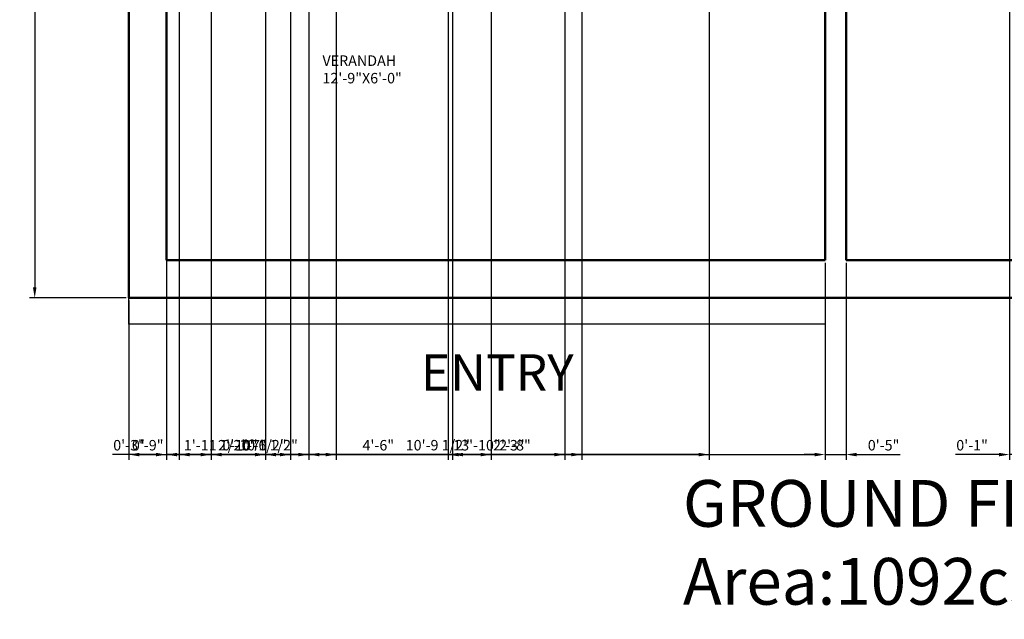
# Model space of a CAD drawing. Units: millimetres. Extents: x 3095 to 3505, y 1097 to 1734.
# Tile 1 of 5: x 3120 to 3355, y 1097 to 1240. Entities that reach past the tile are written whole.
import ezdxf

# ---------------------------------------------------------------- set-up
doc = ezdxf.new("R2010")
doc.units = ezdxf.units.MM
for name, color, linetype, lineweight, true_color in [('A-ANNO-DIMS', 32, 'Continuous', 18, 0xcd6928), ('A-ANNO-TEXT', 152, 'Continuous', 25, 0x2776bb), ('A-AREA-IDEN', 152, 'Continuous', 18, 0x2776bb), ('A-FLOR-STRS', 152, 'Continuous', 25, 0x2776bb)]:
    doc.layers.add(name, color=color, linetype=linetype, lineweight=lineweight, true_color=true_color)
doc.layers.add('A-WALL', color=7, linetype='Continuous', lineweight=50)
doc.styles.get("Standard").update_dxf_attribs({"font": 'arial.ttf'})
doc.dimstyles.new('ISO-25', dxfattribs={"dimtxt": 2.5, "dimasz": 2.5, "dimexe": 1.25, "dimexo": 0.625, "dimtad": 1, "dimlunit": 3, "dimtxsty": 'Standard', "dimcen": 2.5, "dimadec": 0, "dimazin": 0, "dimtfac": 1, "dimtmove": 0, "dimatfit": 3, "dimfxl": 1, "dimarcsym": 0})

# ---------------------------------------------------------------- blocks, each defined once
blk = doc.blocks.new('*D11')
at = {"layer": 'A-ANNO-DIMS', "color": 0, "lineweight": -2, "transparency": 16777216}
for p, q in [((3145.24, 1677.32), (3122.17, 1677.32)), ((3123.42, 1674.82), (3123.42, 1175.82)), ((3145.24, 1173.32), (3122.17, 1173.32))]:
    blk.add_line(p, q, dxfattribs=at)
at = {"layer": 'A-ANNO-DIMS', "color": 0, "lineweight": 5, "transparency": 16777216}
for points in [[(3123, 1674.82), (3123.84, 1674.82), (3123.42, 1677.32)], [(3123, 1175.82), (3123.84, 1175.82), (3123.42, 1173.32)]]:
    blk.add_solid(points, dxfattribs=at)
at = {"layer": 'Defpoints', "color": 0, "lineweight": 5, "transparency": 16777216}
for p in [(3145.86, 1677.32), (3123.42, 1173.32), (3145.86, 1173.32)]:
    blk.add_point(p, dxfattribs=at)
at = {"layer": 'A-ANNO-DIMS', "color": 0, "transparency": 16777216, "insert": (3121.54, 1425.32), "char_height": 2.5, "attachment_point": 5, "rotation": 90}
blk.add_mtext("42'", dxfattribs=at)
blk = doc.blocks.new('*D43')
at = {"layer": 'A-ANNO-DIMS', "color": 0, "lineweight": -2, "transparency": 16777216}
for p, q in [((3154.86, 1181.69), (3154.86, 1134.75)), ((3145.86, 1172.69), (3145.86, 1134.75)), ((3148.36, 1136), (3152.36, 1136))]:
    blk.add_line(p, q, dxfattribs=at)
at = {"layer": 'A-ANNO-DIMS', "color": 0, "lineweight": 5, "transparency": 16777216}
for points in [[(3148.36, 1136.41), (3148.36, 1135.58), (3145.86, 1136)], [(3152.36, 1136.41), (3152.36, 1135.58), (3154.86, 1136)]]:
    blk.add_solid(points, dxfattribs=at)
at = {"layer": 'Defpoints', "color": 0, "lineweight": 5, "transparency": 16777216}
for p in [(3154.86, 1182.32), (3145.86, 1173.32), (3154.86, 1136)]:
    blk.add_point(p, dxfattribs=at)
at = {"layer": 'A-ANNO-DIMS', "color": 0, "transparency": 16777216, "insert": (3150.36, 1137.9), "char_height": 2.5, "attachment_point": 5}
blk.add_mtext('0\'-9"', dxfattribs=at)
blk = doc.blocks.new('*D44')
at = {"layer": 'A-ANNO-DIMS', "color": 0, "lineweight": -2, "transparency": 16777216}
for p, q in [((3311.86, 1181.69), (3311.86, 1134.75)), ((3316.86, 1181.69), (3316.86, 1134.75)), ((3309.36, 1136), (3306.86, 1136)), ((3311.86, 1136), (3316.86, 1136)), ((3319.36, 1136), (3329.76, 1136))]:
    blk.add_line(p, q, dxfattribs=at)
at = {"layer": 'A-ANNO-DIMS', "color": 0, "lineweight": 5, "transparency": 16777216}
for points in [[(3309.36, 1136.41), (3309.36, 1135.58), (3311.86, 1136)], [(3319.36, 1136.41), (3319.36, 1135.58), (3316.86, 1136)]]:
    blk.add_solid(points, dxfattribs=at)
at = {"layer": 'Defpoints', "color": 0, "lineweight": 5, "transparency": 16777216}
for p in [(3311.86, 1182.32), (3316.86, 1182.32), (3316.86, 1136)]:
    blk.add_point(p, dxfattribs=at)
at = {"layer": 'A-ANNO-DIMS', "color": 0, "transparency": 16777216, "insert": (3325.81, 1137.9), "char_height": 2.5, "attachment_point": 5}
blk.add_mtext('0\'-5"', dxfattribs=at)
blk = doc.blocks.new('*D49')
at = {"layer": 'A-ANNO-DIMS', "color": 0, "lineweight": -2, "transparency": 16777216}
for p, q in [((3154.86, 1588.17), (3154.86, 1134.75)), ((3188.81, 1588.17), (3188.81, 1134.75)), ((3157.36, 1136), (3186.31, 1136))]:
    blk.add_line(p, q, dxfattribs=at)
at = {"layer": 'A-ANNO-DIMS', "color": 0, "lineweight": 5, "transparency": 16777216}
for points in [[(3157.36, 1136.41), (3157.36, 1135.58), (3154.86, 1136)], [(3186.31, 1136.41), (3186.31, 1135.58), (3188.81, 1136)]]:
    blk.add_solid(points, dxfattribs=at)
at = {"layer": 'Defpoints', "color": 0, "lineweight": 5, "transparency": 16777216}
for p in [(3154.86, 1588.8), (3188.81, 1588.8), (3188.81, 1136)]:
    blk.add_point(p, dxfattribs=at)
at = {"layer": 'A-ANNO-DIMS', "color": 0, "transparency": 16777216, "insert": (3171.84, 1137.9), "char_height": 2.5, "attachment_point": 5}
blk.add_mtext('2\'-10"', dxfattribs=at)
blk = doc.blocks.new('*D50')
at = {"layer": 'A-ANNO-DIMS', "color": 0, "lineweight": -2, "transparency": 16777216}
for p, q in [((3222, 1588.17), (3222, 1134.75)), ((3253.86, 1588.17), (3253.86, 1134.75)), ((3224.5, 1136), (3251.36, 1136))]:
    blk.add_line(p, q, dxfattribs=at)
at = {"layer": 'A-ANNO-DIMS', "color": 0, "lineweight": 5, "transparency": 16777216}
for points in [[(3224.5, 1136.41), (3224.5, 1135.58), (3222, 1136)], [(3251.36, 1136.41), (3251.36, 1135.58), (3253.86, 1136)]]:
    blk.add_solid(points, dxfattribs=at)
at = {"layer": 'Defpoints', "color": 0, "lineweight": 5, "transparency": 16777216}
for p in [(3222, 1588.8), (3253.86, 1588.8), (3253.86, 1136)]:
    blk.add_point(p, dxfattribs=at)
at = {"layer": 'A-ANNO-DIMS', "color": 0, "transparency": 16777216, "insert": (3237.93, 1137.9), "char_height": 2.5, "attachment_point": 5}
blk.add_mtext('2\'-8"', dxfattribs=at)
blk = doc.blocks.new('*D52')
at = {"layer": 'A-ANNO-DIMS', "color": 0, "lineweight": -2, "transparency": 16777216}
for p, q in [((3178.42, 1456.63), (3178.42, 1134.75)), ((3232.26, 1456.63), (3232.26, 1134.75)), ((3180.92, 1136), (3229.76, 1136))]:
    blk.add_line(p, q, dxfattribs=at)
at = {"layer": 'A-ANNO-DIMS', "color": 0, "lineweight": 5, "transparency": 16777216}
for points in [[(3180.92, 1136.41), (3180.92, 1135.58), (3178.42, 1136)], [(3229.76, 1136.41), (3229.76, 1135.58), (3232.26, 1136)]]:
    blk.add_solid(points, dxfattribs=at)
at = {"layer": 'Defpoints', "color": 0, "lineweight": 5, "transparency": 16777216}
for p in [(3178.42, 1457.25), (3232.26, 1457.25), (3232.26, 1136)]:
    blk.add_point(p, dxfattribs=at)
at = {"layer": 'A-ANNO-DIMS', "color": 0, "transparency": 16777216, "insert": (3205.34, 1137.9), "char_height": 2.5, "attachment_point": 5}
blk.add_mtext('4\'-6"', dxfattribs=at)
blk = doc.blocks.new('*D57')
at = {"layer": 'A-ANNO-DIMS', "color": 0, "lineweight": -2, "transparency": 16777216}
for p, q in [((3165.47, 1598.31), (3165.47, 1134.75)), ((3184.42, 1598.31), (3184.42, 1134.75)), ((3167.97, 1136), (3181.92, 1136))]:
    blk.add_line(p, q, dxfattribs=at)
at = {"layer": 'A-ANNO-DIMS', "color": 0, "lineweight": 5, "transparency": 16777216}
for points in [[(3167.97, 1136.41), (3167.97, 1135.58), (3165.47, 1136)], [(3181.92, 1136.41), (3181.92, 1135.58), (3184.42, 1136)]]:
    blk.add_solid(points, dxfattribs=at)
at = {"layer": 'Defpoints', "color": 0, "lineweight": 5, "transparency": 16777216}
for p in [(3165.47, 1598.93), (3184.42, 1598.93), (3184.42, 1136)]:
    blk.add_point(p, dxfattribs=at)
at = {"layer": 'A-ANNO-DIMS', "color": 0, "transparency": 16777216, "insert": (3174.95, 1137.88), "char_height": 2.5, "attachment_point": 5}
blk.add_mtext('1\'-7"', dxfattribs=at)
blk = doc.blocks.new('*D64')
at = {"layer": 'A-ANNO-DIMS', "color": 0, "lineweight": -2, "transparency": 16777216}
for p, q in [((3355.86, 1317.69), (3355.86, 1134.75)), ((3356.76, 1312.81), (3356.76, 1134.75)), ((3353.36, 1136), (3342.97, 1136)), ((3356.76, 1136), (3355.86, 1136)), ((3359.26, 1136), (3361.76, 1136))]:
    blk.add_line(p, q, dxfattribs=at)
at = {"layer": 'A-ANNO-DIMS', "color": 0, "lineweight": 5, "transparency": 16777216}
for points in [[(3353.36, 1136.41), (3353.36, 1135.58), (3355.86, 1136)], [(3359.26, 1136.41), (3359.26, 1135.58), (3356.76, 1136)]]:
    blk.add_solid(points, dxfattribs=at)
at = {"layer": 'Defpoints', "color": 0, "lineweight": 5, "transparency": 16777216}
for p in [(3355.86, 1318.32), (3356.76, 1313.43), (3355.86, 1136)]:
    blk.add_point(p, dxfattribs=at)
at = {"layer": 'A-ANNO-DIMS', "color": 0, "transparency": 16777216, "insert": (3346.91, 1137.9), "char_height": 2.5, "attachment_point": 5}
blk.add_mtext('0\'-1"', dxfattribs=at)
blk = doc.blocks.new('*D65')
at = {"layer": 'A-ANNO-DIMS', "color": 0, "lineweight": -2, "transparency": 16777216}
for p, q in [((3178.42, 1456.63), (3178.42, 1134.75)), ((3154.86, 1439.69), (3154.86, 1134.75)), ((3175.92, 1136), (3157.36, 1136))]:
    blk.add_line(p, q, dxfattribs=at)
at = {"layer": 'A-ANNO-DIMS', "color": 0, "lineweight": 5, "transparency": 16777216}
for points in [[(3157.36, 1136.41), (3157.36, 1135.58), (3154.86, 1136)], [(3175.92, 1136.41), (3175.92, 1135.58), (3178.42, 1136)]]:
    blk.add_solid(points, dxfattribs=at)
at = {"layer": 'Defpoints', "color": 0, "lineweight": 5, "transparency": 16777216}
for p in [(3178.42, 1457.25), (3154.86, 1440.32), (3154.86, 1136)]:
    blk.add_point(p, dxfattribs=at)
at = {"layer": 'A-ANNO-DIMS', "color": 0, "transparency": 16777216, "insert": (3166.64, 1137.91), "char_height": 2.5, "attachment_point": 5}
blk.add_mtext('1\'-11 1/2"', dxfattribs=at)
blk = doc.blocks.new('*D67')
at = {"layer": 'A-ANNO-DIMS', "color": 0, "lineweight": -2, "transparency": 16777216}
for p, q in [((3154.86, 1253.69), (3154.86, 1134.75)), ((3284.21, 1253.69), (3284.21, 1134.75)), ((3281.71, 1136), (3157.36, 1136))]:
    blk.add_line(p, q, dxfattribs=at)
at = {"layer": 'A-ANNO-DIMS', "color": 0, "lineweight": 5, "transparency": 16777216}
for points in [[(3157.36, 1136.41), (3157.36, 1135.58), (3154.86, 1136)], [(3281.71, 1136.41), (3281.71, 1135.58), (3284.21, 1136)]]:
    blk.add_solid(points, dxfattribs=at)
at = {"layer": 'Defpoints', "color": 0, "lineweight": 5, "transparency": 16777216}
for p in [(3154.86, 1254.32), (3284.21, 1254.31), (3154.86, 1136)]:
    blk.add_point(p, dxfattribs=at)
at = {"layer": 'A-ANNO-DIMS', "color": 0, "transparency": 16777216, "insert": (3219.53, 1137.91), "char_height": 2.5, "attachment_point": 5}
blk.add_mtext('10\'-9 1/2"', dxfattribs=at)
blk = doc.blocks.new('*D68')
at = {"layer": 'A-ANNO-DIMS', "color": 0, "lineweight": -2, "transparency": 16777216}
for p, q in [((3223.06, 1317.18), (3223.06, 1134.75)), ((3249.85, 1317.18), (3249.85, 1134.75)), ((3225.56, 1136), (3247.35, 1136))]:
    blk.add_line(p, q, dxfattribs=at)
at = {"layer": 'A-ANNO-DIMS', "color": 0, "lineweight": 5, "transparency": 16777216}
for points in [[(3225.56, 1136.41), (3225.56, 1135.58), (3223.06, 1136)], [(3247.35, 1136.41), (3247.35, 1135.58), (3249.85, 1136)]]:
    blk.add_solid(points, dxfattribs=at)
at = {"layer": 'Defpoints', "color": 0, "lineweight": 5, "transparency": 16777216}
for p in [(3223.06, 1317.8), (3249.85, 1317.8), (3249.85, 1136)]:
    blk.add_point(p, dxfattribs=at)
at = {"layer": 'A-ANNO-DIMS', "color": 0, "transparency": 16777216, "insert": (3236.46, 1137.9), "char_height": 2.5, "attachment_point": 5}
blk.add_mtext('2\'-3"', dxfattribs=at)
blk = doc.blocks.new('*D70')
at = {"layer": 'A-ANNO-DIMS', "color": 0, "lineweight": -2, "transparency": 16777216}
for p, q in [((3165.47, 1598.31), (3165.47, 1134.75)), ((3154.86, 1588.17), (3154.86, 1134.75)), ((3157.36, 1136), (3162.97, 1136)), ((3165.47, 1136), (3183.64, 1136))]:
    blk.add_line(p, q, dxfattribs=at)
at = {"layer": 'A-ANNO-DIMS', "color": 0, "lineweight": 5, "transparency": 16777216}
for points in [[(3157.36, 1136.41), (3157.36, 1135.58), (3154.86, 1136)], [(3162.97, 1136.41), (3162.97, 1135.58), (3165.47, 1136)]]:
    blk.add_solid(points, dxfattribs=at)
at = {"layer": 'Defpoints', "color": 0, "lineweight": 5, "transparency": 16777216}
for p in [(3165.47, 1598.93), (3154.86, 1588.8), (3165.47, 1136)]:
    blk.add_point(p, dxfattribs=at)
at = {"layer": 'A-ANNO-DIMS', "color": 0, "transparency": 16777216, "insert": (3175.81, 1137.91), "char_height": 2.5, "attachment_point": 5}
blk.add_mtext('0\'-10 1/2"', dxfattribs=at)
blk = doc.blocks.new('*D72')
at = {"layer": 'A-ANNO-DIMS', "color": 0, "lineweight": -2, "transparency": 16777216}
for p, q in [((3195.33, 1651.97), (3195.33, 1134.75)), ((3188.81, 1649.1), (3188.81, 1134.75)), ((3188.81, 1136), (3172.59, 1136)), ((3192.83, 1136), (3191.31, 1136))]:
    blk.add_line(p, q, dxfattribs=at)
at = {"layer": 'A-ANNO-DIMS', "color": 0, "lineweight": 5, "transparency": 16777216}
for points in [[(3191.31, 1136.41), (3191.31, 1135.58), (3188.81, 1136)], [(3192.83, 1136.41), (3192.83, 1135.58), (3195.33, 1136)]]:
    blk.add_solid(points, dxfattribs=at)
at = {"layer": 'Defpoints', "color": 0, "lineweight": 5, "transparency": 16777216}
for p in [(3195.33, 1652.6), (3188.81, 1649.73), (3188.81, 1136)]:
    blk.add_point(p, dxfattribs=at)
at = {"layer": 'A-ANNO-DIMS', "color": 0, "transparency": 16777216, "insert": (3179.45, 1137.91), "char_height": 2.5, "attachment_point": 5}
blk.add_mtext('0\'-6 1/2"', dxfattribs=at)
blk = doc.blocks.new('*D74')
at = {"layer": 'A-ANNO-DIMS', "color": 0, "lineweight": -2, "transparency": 16777216}
for p, q in [((3157.86, 1274.09), (3157.86, 1134.75)), ((3154.86, 1258.69), (3154.86, 1134.75)), ((3152.36, 1136), (3141.97, 1136)), ((3157.86, 1136), (3154.86, 1136)), ((3160.36, 1136), (3162.86, 1136))]:
    blk.add_line(p, q, dxfattribs=at)
at = {"layer": 'A-ANNO-DIMS', "color": 0, "lineweight": 5, "transparency": 16777216}
for points in [[(3152.36, 1136.41), (3152.36, 1135.58), (3154.86, 1136)], [(3160.36, 1136.41), (3160.36, 1135.58), (3157.86, 1136)]]:
    blk.add_solid(points, dxfattribs=at)
at = {"layer": 'Defpoints', "color": 0, "lineweight": 5, "transparency": 16777216}
for p in [(3157.86, 1274.71), (3154.86, 1259.32), (3154.86, 1136)]:
    blk.add_point(p, dxfattribs=at)
at = {"layer": 'A-ANNO-DIMS', "color": 0, "transparency": 16777216, "insert": (3145.91, 1137.9), "char_height": 2.5, "attachment_point": 5}
blk.add_mtext('0\'-3"', dxfattribs=at)
blk = doc.blocks.new('*D80')
at = {"layer": 'A-ANNO-DIMS', "color": 0, "lineweight": -2, "transparency": 16777216}
for p, q in [((3145.86, 1172.69), (3145.86, 1134.75)), ((3311.86, 1172.69), (3311.86, 1134.75)), ((3148.36, 1136), (3309.36, 1136))]:
    blk.add_line(p, q, dxfattribs=at)
at = {"layer": 'A-ANNO-DIMS', "color": 0, "lineweight": 5, "transparency": 16777216}
for points in [[(3148.36, 1136.41), (3148.36, 1135.58), (3145.86, 1136)], [(3309.36, 1136.41), (3309.36, 1135.58), (3311.86, 1136)]]:
    blk.add_solid(points, dxfattribs=at)
at = {"layer": 'Defpoints', "color": 0, "lineweight": 5, "transparency": 16777216}
for p in [(3145.86, 1173.32), (3311.86, 1173.32), (3311.86, 1136)]:
    blk.add_point(p, dxfattribs=at)
at = {"layer": 'A-ANNO-DIMS', "color": 0, "transparency": 16777216, "insert": (3228.86, 1137.9), "char_height": 2.5, "attachment_point": 5}
blk.add_mtext('13\'-10"', dxfattribs=at)

msp = doc.modelspace()

# ---------------------------------------------------------------- linework, layer by layer
at = {"layer": 'A-FLOR-STRS'}
msp.add_lwpolyline([(3145.862, 1173.316), (3311.862, 1173.316), (3311.862, 1167.046), (3145.862, 1167.046)], close=True, dxfattribs=at)
at = {"layer": 'A-WALL'}
for p, q in [((3145.862, 1173.316), (3145.862, 1677.316)), ((3316.862, 1313.316), (3316.862, 1182.316)), ((3154.862, 1182.316), (3154.862, 1254.316)), ((3311.862, 1254.316), (3311.862, 1182.316)), ((3311.862, 1182.316), (3154.862, 1182.316)), ((3448.862, 1182.316), (3316.862, 1182.316)), ((3457.862, 1173.316), (3145.862, 1173.316))]:
    msp.add_line(p, q, dxfattribs=at)

# ---------------------------------------------------------------- texts
at = {"layer": 'A-ANNO-TEXT', "attachment_point": 1}
for s, width, gutter_width, insert, char_height in [('ENTRY', 164.49923, 43.399, (3215.489, 1159.894), 8.6799), ('GROUND FLOOR PLAN\\PArea:1092csq.ft', 1117.06792, 55.702, (3277.968, 1129.938), 11.14035)]:
    msp.add_mtext_dynamic_manual_height_columns(s, width=width, gutter_width=gutter_width, heights=[0], dxfattribs=dict(at, insert=insert, char_height=char_height))
at = {"layer": 'A-AREA-IDEN', "insert": (3192.029, 1231.116), "char_height": 2.5, "attachment_point": 1}
msp.add_mtext_dynamic_manual_height_columns('VERANDAH\\P12\'-9"X6\'-0"', width=55.13342, gutter_width=12.5, heights=[0], dxfattribs=at)

# ---------------------------------------------------------------- dimensions: what is measured, and where the dimension line sits
at = {"layer": 'A-ANNO-DIMS'}
dim = msp.add_linear_dim(base=(3123.421, 1173.316), p1=(3145.862, 1677.316), p2=(3145.862, 1173.316), angle=90, dimstyle='ISO-25', override={"dimclrd": 0, "dimclre": 0, "dimclrt": 0}, dxfattribs=at)
dim.commit()
dim.dimension.update_dxf_attribs({"geometry": '*D11', "text_midpoint": (3121.541, 1425.316)})
for base, p1, p2, picture, middle in [((3188.808, 1135.996), (3195.33, 1652.599), (3188.808, 1649.727), '*D72', (3179.447, 1137.914)), ((3165.474, 1135.996), (3154.862, 1588.796), (3165.474, 1598.93), '*D70', (3175.806, 1137.914)), ((3184.422, 1135.996), (3165.474, 1598.93), (3184.422, 1598.93), '*D57', (3174.948, 1137.877)), ((3188.808, 1135.996), (3154.862, 1588.796), (3188.808, 1588.796), '*D49', (3171.835, 1137.898)), ((3253.862, 1135.996), (3221.995, 1588.796), (3253.862, 1588.796), '*D50', (3237.929, 1137.898)), ((3154.862, 1135.996), (3178.42, 1457.251), (3154.862, 1440.316), '*D65', (3166.641, 1137.914)), ((3232.262, 1135.996), (3178.42, 1457.251), (3232.262, 1457.251), '*D52', (3205.341, 1137.898)), ((3249.851, 1135.996), (3223.059, 1317.802), (3249.851, 1317.802), '*D68', (3236.455, 1137.899)), ((3355.862, 1135.996), (3356.756, 1313.435), (3355.862, 1318.316), '*D64', (3346.915, 1137.898)), ((3154.862, 1135.996), (3157.862, 1274.711), (3154.862, 1259.316), '*D74', (3145.915, 1137.899)), ((3154.862, 1135.996), (3284.206, 1254.31), (3154.862, 1254.316), '*D67', (3219.534, 1137.914)), ((3154.862, 1135.996), (3145.862, 1173.316), (3154.862, 1182.316), '*D43', (3150.362, 1137.898)), ((3316.862, 1135.996), (3311.862, 1182.316), (3316.862, 1182.316), '*D44', (3325.81, 1137.898)), ((3311.862, 1135.996), (3145.862, 1173.316), (3311.862, 1173.316), '*D80', (3228.862, 1137.899))]:
    dim = msp.add_linear_dim(base=base, p1=p1, p2=p2, dimstyle='ISO-25', override={"dimdec": 1, "dimlfac": 1, "dimrnd": 0, "dimzin": 1, "dimdsep": 46, "dimlunit": 4, "dimfrac": 2}, dxfattribs=at)
    dim.commit()
    dim.dimension.update_dxf_attribs({"geometry": picture, "text_midpoint": middle})

doc.saveas('drawing.dxf')
